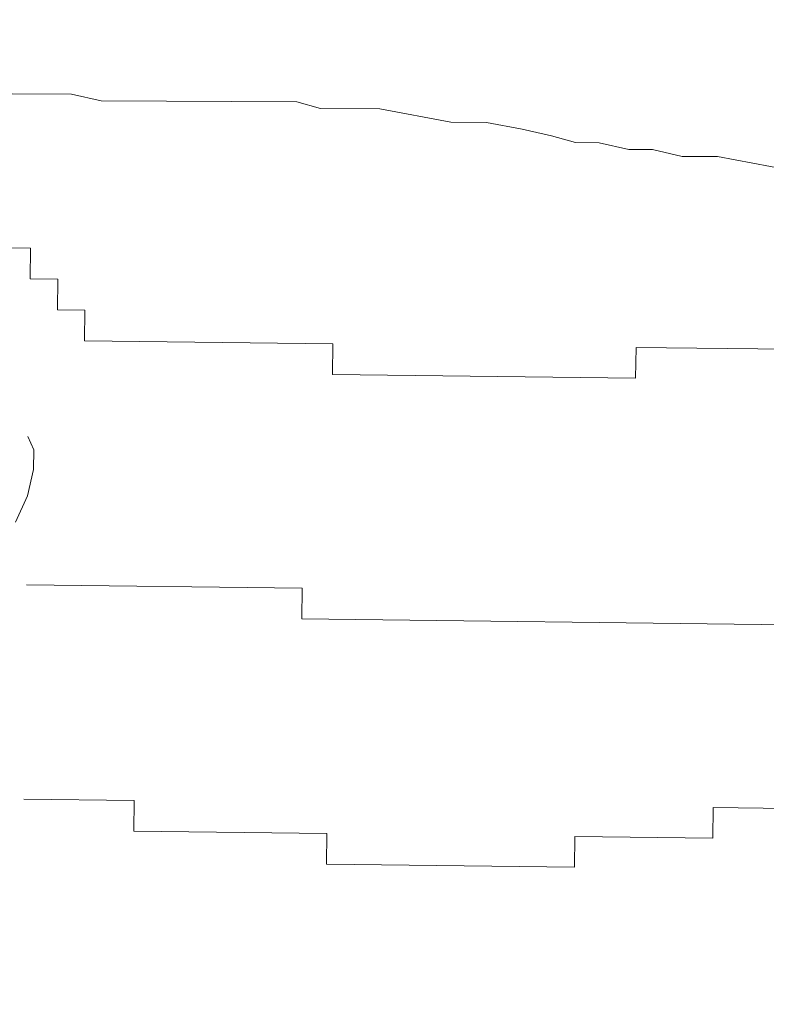
# Model space of a CAD drawing. Units: inches. Extents: x -466983 to 1020, y 324 to 318697.
# Tile 78 of 97: x 652.867 to 656.235, y 944.271 to 948.713. Entities that reach past the tile are written whole.
import ezdxf

# ---------------------------------------------------------------- set-up
doc = ezdxf.new("R2010")
doc.units = ezdxf.units.IN
doc.header["$MEASUREMENT"] = 0
doc.layers.add('A-FLOR-PATT', color=252, linetype='Continuous', lineweight=13)
doc.layers.add('A-FURN', color=8, linetype='Continuous', lineweight=18)

# ---------------------------------------------------------------- blocks, each defined once
blk = doc.blocks.new('L Shaped Sofa')
at = {"ltscale": 2}
for p, q in [((2397.618, 739.4823), (2397.6211, 739.7342)), ((2397.6211, 739.7342), (2399.6627, 739.7093)), ((2399.6627, 739.7093), (2399.6596, 739.4574)), ((2396.4808, 739.2443), (2396.4839, 739.4962)), ((2396.4839, 739.4962), (2397.618, 739.4823)), ((2399.6596, 739.4574), (2401.2474, 739.438)), ((2401.2474, 739.438), (2401.2444, 739.1861)), ((2393.5319, 739.2803), (2396.4808, 739.2443)), ((2401.2444, 739.1861), (2402.1517, 739.175)), ((2395.555, 737.7439), (2399.8649, 737.6912)), ((2399.8649, 737.6912), (2399.8618, 737.4393)), ((2399.8618, 737.4393), (2402.1302, 737.4116)), ((2402.1214, 736.6787), (2402.2204, 736.8951)), ((2402.0713, 736.4621), (2402.1214, 736.6787)), ((2402.0703, 736.2994), (2402.0713, 736.4621)), ((2402.1185, 736.1908), (2402.0703, 736.2994)), ((2397.1151, 735.4573), (2397.1182, 735.7092)), ((2397.1182, 735.7092), (2399.6134, 735.6787)), ((2399.6134, 735.6787), (2399.6103, 735.4268)), ((2394.6199, 735.4878), (2397.1151, 735.4573)), ((2399.6103, 735.4268), (2401.6519, 735.4018)), ((2401.6519, 735.4018), (2401.6488, 735.1499)), ((2401.6488, 735.1499), (2401.8756, 735.1472)), ((2401.8756, 735.1472), (2401.8725, 734.8952)), ((2401.8725, 734.8952), (2402.0994, 734.8925)), ((2402.0994, 734.8925), (2402.0963, 734.6406)), ((2402.0963, 734.6406), (2402.3231, 734.6378)), ((2395.8591, 733.9972), (2396.444, 733.8861)), ((2396.444, 733.8861), (2396.7367, 733.8847)), ((2396.7367, 733.8847), (2396.9804, 733.8293)), ((2396.9804, 733.8293), (2397.1755, 733.8284)), ((2397.1755, 733.8284), (2397.4192, 733.7731)), ((2397.4192, 733.7731), (2397.6144, 733.7721)), ((2397.6144, 733.7721), (2397.8092, 733.717)), ((2397.8092, 733.717), (2398.0529, 733.6616)), ((2398.0529, 733.6616), (2398.3453, 733.6061)), ((2398.3453, 733.6061), (2398.6381, 733.6047)), ((2398.6381, 733.6047), (2399.223, 733.4935)), ((2399.223, 733.4935), (2399.7109, 733.4912)), ((2399.7109, 733.4912), (2399.9058, 733.4361)), ((2399.9058, 733.4361), (2401.516, 733.4285)), ((2401.516, 733.4285), (2401.7596, 733.3732)), ((2401.7596, 733.3732), (2402.2476, 733.3709))]:
    blk.add_line(p, q, dxfattribs=at)

msp = doc.modelspace()

# ---------------------------------------------------------------- hatches: boundary and pattern name
at = {"layer": 'A-FLOR-PATT', "transparency": 33554572}
h = msp.add_hatch(dxfattribs=at)
h.set_pattern_fill('ANSI37', color=256, scale=30)
h.set_pattern_definition([(45, (-1212.4137, -290.035), (-2.6516504, 2.6516504), []), (135, (-1212.4137, -290.035), (-2.6516504, -2.6516504), [])])
h.paths.add_polyline_path([(901.8057, 1075.9377), (900.6144, 1075.9377), (900.6144, 1065.3856), (899.391, 1065.3856), (898.0911, 1065.3856), (892.8356, 1058.7098, -0.258377), (892.1875, 1058.3509), (879.9848, 1058.3509, -0.20177), (879.4382, 1058.5808), (874.0812, 1065.3856), (872.7813, 1065.3856), (871.5579, 1065.3856), (871.5579, 1075.9377), (813.8057, 1075.9377), (813.8057, 1044.7922), (832.3947, 1044.7922, -0.394795), (848.6602, 1028.5356), (848.6602, 1009.9377), (901.8057, 1009.9377), (901.8057, 1015.9377), (901.3057, 1015.9377), (871.3057, 1015.9377), (871.3057, 1017.2502), (871.3344, 1017.2502, -0.401453), (901.3057, 1045.9377), (901.8057, 1045.9377)])
edge = h.paths.add_edge_path(flags=16)
edge.add_line((847.7731, 1068.9486), (847.7731, 1073.7088))
edge.add_arc((849.2269, 1073.7088), 1.4538, 90, 180, ccw=False)
edge.add_line((849.2269, 1075.1627), (864.4921, 1075.1627))
edge.add_arc((864.4921, 1073.7088), 1.4538, 0, 90, ccw=False)
edge.add_line((865.9459, 1073.7088), (865.9459, 1069.0035))
edge.add_arc((832.6447, 1068.9761), 33.3012, -20.61234, 0.04725, ccw=False)
edge.add_ellipse((856.8595, 1058.48), major_axis=(0, 10.2131), ratio=0.6859192, start_angle=100.00884, end_angle=259.99116, ccw=False)
edge.add_arc((881.0742, 1068.9761), 33.3012, 180.04725, 200.61234, ccw=False)
h.paths.add_polyline_path([(853.1456, 1066.4815), (853.1456, 1066.4534), (853.1463, 1066.4534, 0.433107), (852.9166, 1066.6849), (852.9166, 1066.4534), (853.1456, 1066.4534), (853.1456, 1066.4815), (853.088, 1066.6122, 0.697939), (852.6995, 1066.4534), (852.7003, 1066.4534), (852.7003, 1066.4815), (852.9166, 1067.0012), (852.9166, 1066.6849, -0.396254)], flags=0)
h.paths.add_polyline_path([(861.0187, 1066.4815), (861.0187, 1066.4534), (861.0194, 1066.4534, 0.416404), (860.8024, 1066.6849), (860.8024, 1066.4534), (861.0187, 1066.4534), (861.0187, 1066.4815), (860.9672, 1066.6053, 0.713344), (860.5726, 1066.4534), (860.5734, 1066.4534), (860.5734, 1066.4815), (860.8024, 1067.0012), (860.8024, 1066.6849, -0.379973)], flags=0)
edge = h.paths.add_edge_path(flags=0)
edge.add_spline(control_points=[(861.1298, 1065.7855), (861.4661, 1065.2478), (861.6134, 1065.0161), (861.9833, 1064.3736), (862.1924, 1063.9443), (862.5614, 1063.0391), (862.7212, 1062.5633), (862.9865, 1061.5781), (863.092, 1061.0689), (863.2452, 1060.031), (863.293, 1059.5025), (863.3295, 1058.4409), (863.3181, 1057.9078), (863.2366, 1056.8518), (863.1664, 1056.3289), (862.9695, 1055.308), (862.8427, 1054.8099), (862.5365, 1053.8522), (862.3571, 1053.3927), (861.9514, 1052.5249), (861.7251, 1052.1166), (861.233, 1051.3622), (860.9672, 1051.0162), (860.4048, 1050.3949), (860.1082, 1050.1197), (859.4937, 1049.6461), (859.1758, 1049.4476), (858.5276, 1049.1299), (858.1973, 1049.0107), (857.5315, 1048.8518), (857.1959, 1048.8121), (856.5249, 1048.812), (856.1894, 1048.8515), (855.5236, 1049.0101), (855.1933, 1049.1291), (854.545, 1049.4465), (854.2271, 1049.6449), (853.6124, 1050.1183), (853.3158, 1050.3933), (852.7533, 1051.0143), (852.4874, 1051.3602), (851.9952, 1052.1144), (851.7688, 1052.5225), (851.3629, 1053.3902), (851.1834, 1053.8496), (850.877, 1054.8071), (850.7501, 1055.3051), (850.553, 1056.326), (850.4827, 1056.8488), (850.401, 1057.9048), (850.3895, 1058.4379), (850.4257, 1059.4995), (850.4734, 1060.0281), (850.6265, 1061.066), (850.7318, 1061.5753), (850.9969, 1062.5605), (851.1567, 1063.0365), (851.5254, 1063.9418), (851.7345, 1064.3712), (852.1056, 1065.0164), (852.2544, 1065.2503), (852.6082, 1065.7335)], knot_values=[3.915332, 3.915332, 3.915332, 3.915332, 4.013468, 4.013468, 4.175532, 4.175532, 4.337596, 4.337596, 4.49966, 4.49966, 4.661724, 4.661724, 4.823788, 4.823788, 4.985852, 4.985852, 5.147916, 5.147916, 5.30998, 5.30998, 5.472044, 5.472044, 5.634109, 5.634109, 5.796173, 5.796173, 5.958237, 5.958237, 6.120301, 6.120301, 6.282365, 6.282365, 6.444429, 6.444429, 6.606493, 6.606493, 6.768557, 6.768557, 6.930621, 6.930621, 7.092685, 7.092685, 7.254749, 7.254749, 7.416813, 7.416813, 7.578878, 7.578878, 7.740942, 7.740942, 7.903006, 7.903006, 8.06507, 8.06507, 8.227134, 8.227134, 8.389198, 8.389198, 8.551262, 8.551262, 8.65037, 8.65037, 8.65037, 8.65037], degree=3, periodic=0)
edge.add_line((852.6421, 1065.7855), (861.1298, 1065.7855))
edge = h.paths.add_edge_path(flags=0)
edge.add_ellipse((856.8496, 1057.7432), major_axis=(0, 7.7921), ratio=0.687861, start_angle=0, end_angle=360)
h.paths.add_polyline_path([(848.8634, 1069.3891), (848.8634, 1073.9605, -0.414214), (849.9538, 1075.0508), (863.7652, 1075.0508, -0.414214), (864.8555, 1073.9605), (864.8555, 1069.3891, -0.388936), (864.5237, 1069.027, -0.043561), (849.1953, 1069.027, -0.388936)], flags=0)
h.paths.add_polyline_path([(853.1006, 1068.1122, -1), (852.6775, 1068.1122, -1)], flags=0)
edge = h.paths.add_edge_path(flags=0)
edge.add_ellipse((856.8595, 1057.3378), major_axis=(0, 2.207), ratio=0.657164, start_angle=0, end_angle=360)
h.paths.add_polyline_path([(861.0415, 1068.1122, -1), (860.6184, 1068.1122, -1)], flags=0)
edge = h.paths.add_edge_path()
edge.add_line((573.9537, 1057.3412), (573.9537, 1075.9377))
edge.add_line((573.9537, 1075.9377), (558.7308, 1075.9377))
edge.add_line((558.7308, 1075.9377), (558.7308, 1065.3856))
edge.add_line((558.7308, 1065.3856), (557.5074, 1065.3856))
edge.add_line((557.5074, 1065.3856), (556.2075, 1065.3856))
edge.add_line((556.2075, 1065.3856), (550.952, 1058.7098))
edge.add_arc((550.3039, 1059.1155), 0.7646, 270, 327.9483, ccw=False)
edge.add_line((550.3039, 1058.3509), (538.1012, 1058.3509))
edge.add_arc((538.1012, 1059.1155), 0.7646, 224.3704, 270, ccw=False)
edge.add_line((537.5546, 1058.5808), (532.1976, 1065.3856))
edge.add_line((532.1976, 1065.3856), (530.8977, 1065.3856))
edge.add_line((530.8977, 1065.3856), (529.6743, 1065.3856))
edge.add_line((529.6743, 1065.3856), (529.6743, 1075.9377))
edge.add_line((529.6743, 1075.9377), (520.8057, 1075.9377))
edge.add_line((520.8057, 1075.9377), (520.8057, 1045.9377))
edge.add_line((520.8057, 1045.9377), (521.3057, 1045.9377))
edge.add_arc((521.3057, 1015.9377), 30, 2.50749, 90, ccw=False)
edge.add_line((551.277, 1017.2502), (551.3057, 1017.2502))
edge.add_line((551.3057, 1017.2502), (551.3057, 1015.9377))
edge.add_line((551.3057, 1015.9377), (520.8057, 1015.9377))
edge.add_line((520.8057, 1015.9377), (520.8057, 1009.9377))
edge.add_line((520.8057, 1009.9377), (559.1913, 1010.4022))
edge.add_arc((559.1913, 1011.856), 1.4538, 180, 270, ccw=False)
edge.add_line((557.7375, 1011.856), (557.7375, 1016.5613))
edge.add_arc((591.0386, 1016.5888), 33.3012, 159.38766, 180.04725, ccw=False)
edge.add_ellipse((566.8239, 1027.0848), major_axis=(0, 10.2131), ratio=0.6859192, start_angle=280.00884, end_angle=439.99116, ccw=False)
edge.add_arc((542.6091, 1016.5888), 33.3012, 0.04725, 20.61234, ccw=False)
edge.add_line((575.9103, 1016.6162), (575.9103, 1011.856))
edge.add_arc((574.4565, 1011.856), 1.4538, -90, 0, ccw=False)
edge.add_line((574.4565, 1010.4022), (608.8057, 1009.9377))
edge.add_line((608.8057, 1009.9377), (608.8057, 1041.0857))
edge.add_line((608.8057, 1041.0857), (590.2179, 1041.0857))
edge.add_arc((590.775, 1057.9074), 16.8309, 181.92775, 268.10321, ccw=False)
edge = h.paths.add_edge_path()
edge.add_ellipse((494.2443, 583.6204), major_axis=(0, 10.2131), ratio=0.6859192, start_angle=280.00884, end_angle=439.99116, ccw=False)
edge.add_arc((470.0296, 573.1243), 33.3012, 0.04725, 20.61234, ccw=False)
edge.add_line((503.3307, 573.1518), (503.3307, 568.3916))
edge.add_arc((501.8769, 568.3916), 1.4538, -90, 0, ccw=False)
edge.add_line((501.8769, 566.9377), (539.8057, 566.9377))
edge.add_line((539.8057, 566.9377), (539.8057, 572.9377))
edge.add_line((539.8057, 572.9377), (539.3057, 572.9377))
edge.add_line((539.3057, 572.9377), (509.3057, 572.9377))
edge.add_line((509.3057, 572.9377), (509.3057, 574.2502))
edge.add_line((509.3057, 574.2502), (509.3344, 574.2502))
edge.add_arc((539.3057, 572.9377), 30, 90, 177.49251, ccw=False)
edge.add_line((539.3057, 602.9377), (539.8057, 602.9377))
edge.add_line((539.8057, 602.9377), (539.8057, 626.9377))
edge.add_line((539.8057, 626.9377), (531.7718, 626.9377))
edge.add_line((531.7718, 626.9377), (531.7718, 616.3856))
edge.add_line((531.7718, 616.3856), (530.5484, 616.3856))
edge.add_line((530.5484, 616.3856), (529.2485, 616.3856))
edge.add_line((529.2485, 616.3856), (523.7105, 609.3509))
edge.add_line((523.7105, 609.3509), (510.7766, 609.3509))
edge.add_line((510.7766, 609.3509), (505.2386, 616.3856))
edge.add_line((505.2386, 616.3856), (503.9387, 616.3856))
edge.add_line((503.9387, 616.3856), (502.7153, 616.3856))
edge.add_line((502.7153, 616.3856), (502.7153, 626.9377))
edge.add_line((502.7153, 626.9377), (481.6983, 626.9377))
edge.add_line((481.6983, 626.9377), (481.6983, 610.995))
edge.add_arc((467.2703, 611.4728), 14.4359, 271.92775, 358.10321, ccw=False)
edge.add_line((467.7559, 597.0451), (451.8057, 597.0451))
edge.add_line((451.8057, 597.0451), (451.8057, 584.4035))
edge.add_line((451.8057, 584.4035), (451.8057, 566.9377))
edge.add_line((451.8057, 566.9377), (486.6117, 566.9377))
edge.add_arc((486.6117, 568.3916), 1.4538, 180, 270, ccw=False)
edge.add_line((485.1579, 568.3916), (485.1579, 573.0969))
edge.add_arc((518.4591, 573.1243), 33.3012, 159.38766, 180.04725, ccw=False)
h.paths.add_polyline_path([(836.2609, 1020.7328), (879.8898, 1020.7328), (879.8898, 1039.3902), (836.2609, 1039.3902)], flags=25)
h.paths.add_polyline_path([(549.9851, 1036.7492), (593.614, 1036.7492), (593.614, 1055.4065), (549.9851, 1055.4065)], flags=24)
h.paths.add_polyline_path([(475.123, 595.5959), (518.752, 595.5959), (518.752, 614.2532), (475.123, 614.2532)], flags=24)
h = msp.add_hatch(dxfattribs=at)
h.set_pattern_fill('ANSI37', color=256, scale=20)
h.set_pattern_definition([(45, (-1212.4137, -290.035), (-1.767767, 1.767767), []), (135, (-1212.4137, -290.035), (-1.767767, -1.767767), [])])
h.paths.add_polyline_path([(809.8057, 870.9377), (809.8057, 888.1519), (806.9985, 888.1519), (802.6624, 888.1519), (789.3832, 888.1519), (786.2846, 888.1519, -0.414214), (785.4991, 888.9374), (785.4991, 900.1959), (785.4991, 908.4696, -0.414214), (786.8082, 909.7787, -0.414214), (785.4991, 911.0878), (785.4991, 929.1015, -0.414214), (786.8082, 930.4106, -0.414214), (785.4991, 931.7197), (785.4991, 931.9039, -0.414214), (784.19, 930.5948), (766.7223, 930.5948, -0.412359), (765.4132, 931.8956, -0.413741), (764.1145, 930.5782), (744.5781, 930.422, -0.416556), (743.7864, 931.2075), (743.7864, 933.5153), (742.2154, 933.5153), (742.2154, 952.024, -0.001344), (743.7864, 952.1998), (743.7864, 953.9377), (678.5915, 953.9377), (678.5915, 951.1305), (678.5915, 946.7945), (678.5915, 933.5153), (678.5915, 930.4166, -0.414214), (677.806, 929.6312), (666.5475, 929.6312), (658.2738, 929.6312, -0.414214), (656.9647, 930.9403, -0.414214), (655.6556, 929.6312), (637.6419, 929.6312, -0.414214), (636.3328, 930.9403, -0.414214), (635.0237, 929.6312), (634.8395, 929.6312, -0.414214), (636.1486, 928.322), (636.1486, 910.8544, -0.412359), (634.8478, 909.5452, -0.413741), (636.1653, 908.2466), (636.3214, 888.7102, -0.416556), (635.5359, 887.9184), (633.2281, 887.9184), (633.2281, 886.3475), (614.7194, 886.3475, -0.001344), (614.5436, 887.9184), (612.8057, 887.9184), (612.8057, 834.9377), (612.8057, 752.9377), (612.8057, 748.9377), (612.8057, 697.9377), (654.8057, 697.9377), (654.8057, 701.9377), (715.8057, 701.9377), (715.8057, 737.4353), (774.2918, 737.4353), (774.2918, 795.9377), (809.8057, 795.9377)])
h.paths.add_polyline_path([(679.2761, 849.5757, 0.102523), (682.1475, 849.2608, -0.080461), (694.5428, 849.7725, -0.283899), (694.4822, 849.0082, 0.136605), (694.4068, 848.8103, -0.030441), (694.5428, 846.8929), (694.5428, 842.6198), (694.5428, 838.3466, -0.028219), (694.4246, 836.5684), (694.425, 836.5684, 0.196187), (694.4456, 836.2708, -0.302897), (694.5428, 835.467, -0.080461), (682.1475, 835.9787, 0.102523), (679.2761, 835.6638, -0.58611), (678.6457, 836.0169), (678.6457, 849.2227, -0.58611)], flags=16)
h.paths.add_polyline_path([(679.5173, 848.6515, 0.699597), (679.476, 848.6342, 1.20716), (679.1935, 848.7422, 0.010621)], flags=0)
h.paths.add_polyline_path([(679.4923, 836.5608, -0.013798), (679.9178, 836.6594, -0.071703), (682.8533, 837.1434, -0.165743), (682.1665, 839.1006), (682.1665, 842.6094), (682.1665, 846.0603, -0.240616), (683.4733, 848.6767, -0.068263), (693.9295, 849.0082), (693.7875, 848.7083), (693.7875, 849.0228, 0.067332), (683.4733, 848.6767, 0.240616), (682.1665, 846.0603), (682.1665, 842.6094), (682.1665, 839.1006, 0.23459), (683.461, 836.5513, 0.068093), (693.7875, 836.1955), (693.7875, 836.5104), (693.9296, 836.2102, -0.077215), (682.2421, 836.7815, 0.086627), (679.5283, 836.5701, -0.628402), (679.5029, 836.5735), (679.5029, 836.6071, 0.910458)], flags=0)
h.paths.add_polyline_path([(679.476, 848.6364), (679.2069, 848.647), (679.2069, 836.5718, 0.913566), (679.3645, 836.5861), (679.476, 836.5824)], flags=0)
h.paths.add_polyline_path([(679.2761, 829.8604, 0.102523), (682.1475, 829.5455, -0.080461), (694.5428, 830.0572, -0.283899), (694.4822, 829.2929, 0.136605), (694.4068, 829.095, -0.030441), (694.5428, 827.1776), (694.5428, 822.9045), (694.5428, 818.6314, -0.028219), (694.4246, 816.8531), (694.425, 816.8532, 0.196187), (694.4456, 816.5555, -0.302897), (694.5428, 815.7517, -0.080461), (682.1475, 816.2635, 0.102523), (679.2761, 815.9485, -0.58611), (678.6457, 816.3016), (678.6457, 829.5074, -0.58611)], flags=16)
h.paths.add_polyline_path([(679.5173, 828.9362, 0.699597), (679.476, 828.9189, 1.20716), (679.1935, 829.0269, 0.010621)], flags=0)
h.paths.add_polyline_path([(679.4923, 816.8456, -0.013798), (679.9178, 816.9441, -0.071703), (682.8533, 817.4281, -0.165743), (682.1665, 819.3853), (682.1665, 822.8941), (682.1665, 826.345, -0.240616), (683.4733, 828.9614, -0.068263), (693.9295, 829.2929), (693.7875, 828.9931), (693.7875, 829.3076, 0.067332), (683.4733, 828.9614, 0.240616), (682.1665, 826.345), (682.1665, 822.8941), (682.1665, 819.3853, 0.23459), (683.461, 816.836, 0.068093), (693.7875, 816.4802), (693.7875, 816.7952), (693.9296, 816.4949, -0.077215), (682.2421, 817.0662, 0.086627), (679.5283, 816.8549, -0.628402), (679.5029, 816.8582), (679.5029, 816.8918, 0.910458)], flags=0)
h.paths.add_polyline_path([(679.476, 828.9211), (679.2069, 828.9317), (679.2069, 816.8565, 0.913566), (679.3645, 816.8708), (679.476, 816.8671)], flags=0)
h.paths.add_polyline_path([(679.2761, 810.1451, 0.102523), (682.1475, 809.8302, -0.080461), (694.5428, 810.342, -0.3023), (694.4466, 809.5394, 0.10023), (694.4058, 809.3878, -0.03057), (694.5428, 807.4623), (694.5428, 803.1892), (694.5428, 798.9161, -0.03057), (694.4058, 796.9906, 0.10023), (694.4466, 796.839, -0.3023), (694.5428, 796.0365, -0.080461), (682.1475, 796.5482, 0.102523), (679.2761, 796.2333, -0.58611), (678.6457, 796.5863), (678.6457, 809.7921, -0.58611)], flags=16)
h.paths.add_polyline_path([(679.5173, 809.2417, 0.699597), (679.476, 809.2244, 1.20716), (679.1935, 809.3324, 0.010621)], flags=0)
h.paths.add_polyline_path([(679.4923, 797.151, -0.013798), (679.9178, 797.2496, -0.071703), (682.8533, 797.7336, -0.165743), (682.1665, 799.6908), (682.1665, 803.1996), (682.1665, 806.6505, -0.239349), (683.461, 809.2577, -0.072465), (694.4468, 809.5405, 0.197932), (694.425, 809.2405), (693.7875, 809.2985), (693.7875, 809.6135, 0.068093), (683.461, 809.2577, 0.239349), (682.1665, 806.6505), (682.1665, 803.1996), (682.1665, 799.6908, 0.235854), (683.4733, 797.1323, 0.067332), (693.7875, 796.7861), (693.7875, 797.1006), (694.425, 797.1586, 0.197932), (694.4468, 796.8586, -0.080419), (682.1557, 797.3795, 0.083867), (679.5283, 797.1603, -0.628402), (679.5029, 797.1637), (679.5029, 797.1973, 0.910458)], flags=0)
h.paths.add_polyline_path([(679.2069, 809.2372), (679.2069, 797.162, 0.913566), (679.3645, 797.1763), (679.476, 797.1726), (679.476, 809.2266)], flags=0)
h.paths.add_polyline_path([(695.3643, 853.2989), (728.2231, 853.2989), (728.2231, 771.1519), (695.3643, 771.1519)], flags=16)
h.paths.add_polyline_path([(696.0215, 852.6417), (727.5659, 852.6417), (727.5659, 771.809), (696.0215, 771.809)], flags=0)
h.paths.add_polyline_path([(679.2761, 788.7869, 0.102523), (682.1475, 788.472, -0.080461), (694.5428, 788.9837, -0.3023), (694.4466, 788.1812, 0.10023), (694.4058, 788.0296, -0.03057), (694.5428, 786.1041), (694.5428, 781.831), (694.5428, 777.5578, -0.03057), (694.4058, 775.6323, 0.10023), (694.4466, 775.4808, -0.3023), (694.5428, 774.6782, -0.080461), (682.1475, 775.19, 0.102523), (679.2761, 774.875, -0.58611), (678.6457, 775.2281), (678.6457, 788.4339, -0.58611)], flags=16)
h.paths.add_polyline_path([(679.5173, 787.8834, 0.699597), (679.476, 787.8662, 1.20716), (679.1935, 787.9742, 0.010621)], flags=0)
h.paths.add_polyline_path([(679.4923, 775.7928, -0.013798), (679.9178, 775.8914, -0.071703), (682.8533, 776.3753, -0.165743), (682.1665, 778.3325), (682.1665, 781.8414), (682.1665, 785.2922, -0.239349), (683.461, 787.8995, -0.072465), (694.4468, 788.1823, 0.197932), (694.425, 787.8823), (693.7875, 787.9403), (693.7875, 788.2553, 0.068093), (683.461, 787.8995, 0.239349), (682.1665, 785.2922), (682.1665, 781.8414), (682.1665, 778.3325, 0.235854), (683.4733, 775.7741, 0.067332), (693.7875, 775.4279), (693.7875, 775.7424), (694.425, 775.8004, 0.197932), (694.4468, 775.5004, -0.080419), (682.1557, 776.0212, 0.083867), (679.5283, 775.8021, -0.628402), (679.5029, 775.8054), (679.5029, 775.8391, 0.910458)], flags=0)
h.paths.add_polyline_path([(679.2069, 787.8789), (679.2069, 775.8038, 0.913566), (679.3645, 775.818), (679.476, 775.8144), (679.476, 787.8684)], flags=0)
h.paths.add_polyline_path([(704.641, 854.1204, -0.080461), (705.1527, 866.5157, 0.102523), (704.8378, 869.3871, -0.58611), (705.1908, 870.0174), (718.3966, 870.0174, -0.58611), (718.7496, 869.3871, 0.102523), (718.4347, 866.5157, -0.080461), (718.9465, 854.1204, -0.3023), (718.1439, 854.2166, 0.10023), (717.9924, 854.2574, -0.03057), (716.0668, 854.1204), (711.7937, 854.1204), (707.5206, 854.1204, -0.03057), (705.5951, 854.2574, 0.10023), (705.4435, 854.2166, -0.3023)], flags=16)
h.paths.add_polyline_path([(717.8462, 869.1459, 0.699597), (717.8289, 869.1872, 1.20716), (717.9369, 869.4697, 0.010621)], flags=0)
h.paths.add_polyline_path([(705.4631, 854.2164, -0.080419), (705.984, 866.5074, 0.083867), (705.7648, 869.1349, -0.628402), (705.7682, 869.1603), (705.8018, 869.1603, 0.910458), (705.7555, 869.1709, -0.013798), (705.8541, 868.7454, -0.071703), (706.3381, 865.8099, -0.165743), (708.2953, 866.4967), (711.8041, 866.4967), (715.255, 866.4967, -0.239349), (717.8622, 865.2022, -0.072465), (718.145, 854.2164, 0.197932), (717.845, 854.2382), (717.903, 854.8757), (718.218, 854.8757, 0.068093), (717.8622, 865.2022, 0.239349), (715.255, 866.4967), (711.8041, 866.4967), (708.2953, 866.4967, 0.235854), (705.7368, 865.1898, 0.067332), (705.3906, 854.8757), (705.7051, 854.8757), (705.7631, 854.2382, 0.197932)], flags=16)
h.paths.add_polyline_path([(705.7665, 869.4563, 0.913566), (705.7808, 869.2987), (705.7771, 869.1872), (717.8311, 869.1872), (717.8417, 869.4563)], flags=0)
h.paths.add_polyline_path([(729.0446, 842.6198), (729.0446, 846.8929, -0.03057), (729.1817, 848.8184, 0.10023), (729.1408, 848.9699, -0.3023), (729.0446, 849.7725, -0.080461), (741.4399, 849.2608, 0.102523), (744.3113, 849.5757, -0.58611), (744.9417, 849.2227), (744.9417, 836.0169, -0.58611), (744.3113, 835.6638, 0.102523), (741.4399, 835.9787, -0.080461), (729.0446, 835.467, -0.3023), (729.1408, 836.2696, 0.10023), (729.1817, 836.4211, -0.03057), (729.0446, 838.3466)], flags=16)
h.paths.add_polyline_path([(744.1115, 836.5846, 1.20716), (744.3939, 836.4766, 0.010621), (744.0701, 836.5673, 0.699597)], flags=0)
h.paths.add_polyline_path([(729.1407, 836.2684, 0.197932), (729.1624, 836.5684), (729.7999, 836.5104), (729.7999, 836.1955, 0.068093), (740.1264, 836.5513, 0.239349), (741.4209, 839.1585), (741.4209, 842.6094), (741.4209, 846.1182, 0.235854), (740.1141, 848.6767, 0.067332), (729.7999, 849.0228), (729.7999, 848.7083), (729.1624, 848.6503, 0.197932), (729.1407, 848.9504, -0.080419), (741.4317, 848.4295, 0.083867), (744.0591, 848.6486, -0.628402), (744.0845, 848.6453), (744.0845, 848.6117, 0.910458), (744.0951, 848.6579, -0.013798), (743.6696, 848.5594, -0.071703), (740.7341, 848.0754, -0.165743), (741.4209, 846.1182), (741.4209, 842.6094), (741.4209, 839.1585, -0.239349), (740.1264, 836.5513, -0.072465)], flags=0)
h.paths.add_polyline_path([(729.0446, 830.0572, -0.080461), (741.4399, 829.5455, 0.102523), (744.3113, 829.8604, -0.58611), (744.9417, 829.5074), (744.9417, 816.3016, -0.58611), (744.3113, 815.9485, 0.102523), (741.4399, 816.2635, -0.080461), (729.0446, 815.7517, -0.3023), (729.1408, 816.5543, 0.10023), (729.1817, 816.7058, -0.03057), (729.0446, 818.6314), (729.0446, 822.9045), (729.0446, 827.1776, -0.03057), (729.1817, 829.1031, 0.10023), (729.1408, 829.2547, -0.3023)], flags=16)
h.paths.add_polyline_path([(744.1115, 816.8693, 1.20716), (744.3939, 816.7613, 0.010621), (744.0701, 816.852, 0.699597)], flags=0)
h.paths.add_polyline_path([(729.1407, 829.2351, -0.080419), (741.4317, 828.7142, 0.083867), (744.0591, 828.9334, -0.628402), (744.0845, 828.93), (744.0845, 828.8964, 0.910458), (744.0951, 828.9427, -0.013798), (743.6696, 828.8441, -0.071703), (740.7341, 828.3601, -0.165743), (741.4209, 826.4029), (741.4209, 822.8941), (741.4209, 819.4432, -0.239349), (740.1264, 816.836, -0.072465), (729.1407, 816.5531, 0.197932), (729.1624, 816.8532), (729.7999, 816.7952), (729.7999, 816.4802, 0.068093), (740.1264, 816.836, 0.239349), (741.4209, 819.4432), (741.4209, 822.8941), (741.4209, 826.4029, 0.235854), (740.1141, 828.9614, 0.067332), (729.7999, 829.3076), (729.7999, 828.9931), (729.1624, 828.9351, 0.197932)], flags=16)
h.paths.add_polyline_path([(729.0446, 810.342, -0.080461), (741.4399, 809.8302, 0.102523), (744.3113, 810.1451, -0.58611), (744.9417, 809.7921), (744.9417, 796.5863, -0.58611), (744.3113, 796.2333, 0.102523), (741.4399, 796.5482, -0.080461), (729.0446, 796.0365, -0.283899), (729.1052, 796.8007, 0.136605), (729.1806, 796.9987, -0.030441), (729.0446, 798.9161), (729.0446, 803.1892), (729.0446, 807.4623, -0.028219), (729.1628, 809.2406), (729.1624, 809.2405, 0.196187), (729.1418, 809.5382, -0.302897)], flags=16)
h.paths.add_polyline_path([(744.1115, 797.1748, 1.20716), (744.3939, 797.0668, 0.010621), (744.0701, 797.1575, 0.699597)], flags=0)
h.paths.add_polyline_path([(741.3453, 809.0275, 0.086627), (744.0591, 809.2388, -0.628402), (744.0845, 809.2355), (744.0845, 809.2019, 0.910458), (744.0951, 809.2481, -0.013798), (743.6696, 809.1496, -0.071703), (740.7341, 808.6656, -0.165743), (741.4209, 806.7084), (741.4209, 803.1996), (741.4209, 799.7487, -0.240616), (740.1141, 797.1323, -0.068263), (729.658, 796.8008), (729.7999, 797.1006), (729.7999, 796.7861, 0.067332), (740.1141, 797.1323, 0.240616), (741.4209, 799.7487), (741.4209, 803.1996), (741.4209, 806.7084, 0.23459), (740.1264, 809.2577, 0.068093), (729.7999, 809.6135), (729.7999, 809.2985), (729.6578, 809.5988, -0.077215)], flags=0)
h.paths.add_polyline_path([(704.641, 770.3304, -0.283899), (705.4053, 770.2697, 0.136605), (705.6032, 770.1944, -0.030441), (707.5206, 770.3304), (711.7937, 770.3304), (716.0668, 770.3304, -0.028219), (717.8451, 770.2122), (717.845, 770.2126, 0.196187), (718.1427, 770.2331, -0.302897), (718.9465, 770.3304, -0.080461), (718.4347, 757.9351, 0.102523), (718.7496, 755.0637, -0.58611), (718.3966, 754.4333), (705.1908, 754.4333, -0.58611), (704.8378, 755.0637, 0.102523), (705.1527, 757.9351, -0.080461)], flags=16)
h.paths.add_polyline_path([(705.762, 755.3048, 0.699597), (705.7793, 755.2635, 1.20716), (705.6713, 754.9811, 0.010621)], flags=0)
h.paths.add_polyline_path([(705.4053, 769.717), (705.7051, 769.5751), (705.3906, 769.5751, 0.067332), (705.7368, 759.2609, 0.240616), (708.3532, 757.954), (711.8041, 757.954), (715.3129, 757.954, 0.23459), (717.8622, 759.2485, 0.068093), (718.218, 769.5751), (717.903, 769.5751), (718.2033, 769.7172, -0.077215), (717.632, 758.0297, 0.086627), (717.8433, 755.3159, -0.628402), (717.84, 755.2904), (717.8064, 755.2904, 0.910458), (717.8526, 755.2799, -0.013798), (717.7541, 755.7053, -0.071703), (717.2701, 758.6409, -0.165743), (715.3129, 757.954), (711.8041, 757.954), (708.3532, 757.954, -0.240616), (705.7368, 759.2609, -0.068263)], flags=0)
h.paths.add_polyline_path([(729.0446, 788.9837, -0.080461), (741.4399, 788.472, 0.102523), (744.3113, 788.7869, -0.58611), (744.9417, 788.4339), (744.9417, 775.2281, -0.58611), (744.3113, 774.875, 0.102523), (741.4399, 775.19, -0.080461), (729.0446, 774.6782, -0.283899), (729.1052, 775.4425, 0.136605), (729.1806, 775.6405, -0.030441), (729.0446, 777.5578), (729.0446, 781.831), (729.0446, 786.1041, -0.028219), (729.1628, 787.8823), (729.1624, 787.8823, 0.196187), (729.1418, 788.1799, -0.302897)], flags=16)
h.paths.add_polyline_path([(744.1115, 775.8165, 1.20716), (744.3939, 775.7086, 0.010621), (744.0701, 775.7993, 0.699597)], flags=0)
h.paths.add_polyline_path([(741.3453, 787.6692, 0.086627), (744.0591, 787.8806, -0.628402), (744.0845, 787.8773), (744.0845, 787.8437, 0.910458), (744.0951, 787.8899, -0.013798), (743.6696, 787.7913, -0.071703), (740.7341, 787.3074, -0.165743), (741.4209, 785.3502), (741.4209, 781.8414), (741.4209, 778.3905, -0.240616), (740.1141, 775.7741, -0.068263), (729.658, 775.4425), (729.7999, 775.7424), (729.7999, 775.4279, 0.067332), (740.1141, 775.7741, 0.240616), (741.4209, 778.3905), (741.4209, 781.8414), (741.4209, 785.3502, 0.23459), (740.1264, 787.8995, 0.068093), (729.7999, 788.2553), (729.7999, 787.9403), (729.6578, 788.2405, -0.077215)], flags=0)
h.paths.add_polyline_path([(744.1115, 848.6364), (744.1115, 836.5824), (744.3805, 836.5718), (744.3805, 848.647, 0.913566), (744.2229, 848.6327)], flags=0)
h.paths.add_polyline_path([(744.2229, 828.9174), (744.1115, 828.9211), (744.1115, 816.8671), (744.3805, 816.8565), (744.3805, 828.9317, 0.913566)], flags=0)
h.paths.add_polyline_path([(717.8311, 755.2635), (705.7771, 755.2635), (705.7665, 754.9945), (717.8417, 754.9945, 0.913566), (717.8274, 755.1521)], flags=0)
h.paths.add_polyline_path([(744.2229, 809.2229), (744.1115, 809.2266), (744.1115, 797.1726), (744.3805, 797.162), (744.3805, 809.2372, 0.913566)], flags=0)
h.paths.add_polyline_path([(744.1115, 787.8684), (744.1115, 775.8144), (744.3805, 775.8038), (744.3805, 787.8789, 0.913566), (744.2229, 787.8647)], flags=0)
h.paths.add_polyline_path([(678.8774, 877.1228), (737.6127, 877.1228), (737.6127, 899.5116), (678.8774, 899.5116)], flags=24)

# ---------------------------------------------------------------- linework, layer by layer
at = {"layer": 'A-FURN', "ltscale": 2}
for p, q in [((653.1012, 948.3768), (652.8337, 948.378)), ((653.1012, 948.3768), (652.8337, 948.378)), ((653.1012, 948.3768), (652.8337, 948.378)), ((653.1012, 948.3768), (652.8337, 948.378)), ((653.1012, 948.3768), (652.8337, 948.378)), ((653.1012, 948.3768), (652.8337, 948.378)), ((653.2348, 948.3464), (653.1012, 948.3768)), ((653.2348, 948.3464), (653.1012, 948.3768)), ((653.2348, 948.3464), (653.1012, 948.3768)), ((653.2348, 948.3464), (653.1012, 948.3768)), ((653.2348, 948.3464), (653.1012, 948.3768)), ((653.2348, 948.3464), (653.1012, 948.3768)), ((654.1176, 948.3423), (653.2348, 948.3464)), ((654.1176, 948.3423), (653.2348, 948.3464)), ((654.1176, 948.3423), (653.2348, 948.3464)), ((654.1176, 948.3423), (653.2348, 948.3464)), ((654.1176, 948.3423), (653.2348, 948.3464)), ((654.1176, 948.3423), (653.2348, 948.3464)), ((654.2244, 948.3121), (654.1176, 948.3423)), ((654.2244, 948.3121), (654.1176, 948.3423)), ((654.2244, 948.3121), (654.1176, 948.3423)), ((654.2244, 948.3121), (654.1176, 948.3423)), ((654.2244, 948.3121), (654.1176, 948.3423)), ((654.2244, 948.3121), (654.1176, 948.3423)), ((654.4919, 948.3108), (654.2244, 948.3121)), ((654.4919, 948.3108), (654.2244, 948.3121)), ((654.4919, 948.3108), (654.2244, 948.3121)), ((654.4919, 948.3108), (654.2244, 948.3121)), ((654.4919, 948.3108), (654.2244, 948.3121)), ((654.4919, 948.3108), (654.2244, 948.3121)), ((654.8125, 948.2498), (654.4919, 948.3108)), ((654.8125, 948.2498), (654.4919, 948.3108)), ((654.8125, 948.2498), (654.4919, 948.3108)), ((654.8125, 948.2498), (654.4919, 948.3108)), ((654.8125, 948.2498), (654.4919, 948.3108)), ((654.8125, 948.2498), (654.4919, 948.3108)), ((654.973, 948.2491), (654.8125, 948.2498)), ((654.973, 948.2491), (654.8125, 948.2498)), ((654.973, 948.2491), (654.8125, 948.2498)), ((654.973, 948.2491), (654.8125, 948.2498)), ((654.973, 948.2491), (654.8125, 948.2498)), ((654.973, 948.2491), (654.8125, 948.2498)), ((655.1334, 948.2186), (654.973, 948.2491)), ((655.1334, 948.2186), (654.973, 948.2491)), ((655.1334, 948.2186), (654.973, 948.2491)), ((655.1334, 948.2186), (654.973, 948.2491)), ((655.1334, 948.2186), (654.973, 948.2491)), ((655.1334, 948.2186), (654.973, 948.2491)), ((655.2669, 948.1883), (655.1334, 948.2186)), ((655.2669, 948.1883), (655.1334, 948.2186)), ((655.2669, 948.1883), (655.1334, 948.2186)), ((655.2669, 948.1883), (655.1334, 948.2186)), ((655.2669, 948.1883), (655.1334, 948.2186)), ((655.2669, 948.1883), (655.1334, 948.2186)), ((655.3737, 948.158), (655.2669, 948.1883)), ((655.3737, 948.158), (655.2669, 948.1883)), ((655.3737, 948.158), (655.2669, 948.1883)), ((655.3737, 948.158), (655.2669, 948.1883)), ((655.3737, 948.158), (655.2669, 948.1883)), ((655.3737, 948.158), (655.2669, 948.1883)), ((655.4807, 948.1575), (655.3737, 948.158)), ((655.4807, 948.1575), (655.3737, 948.158)), ((655.4807, 948.1575), (655.3737, 948.158)), ((655.4807, 948.1575), (655.3737, 948.158)), ((655.4807, 948.1575), (655.3737, 948.158)), ((655.4807, 948.1575), (655.3737, 948.158)), ((655.6143, 948.1272), (655.4807, 948.1575)), ((655.6143, 948.1272), (655.4807, 948.1575)), ((655.6143, 948.1272), (655.4807, 948.1575)), ((655.6143, 948.1272), (655.4807, 948.1575)), ((655.6143, 948.1272), (655.4807, 948.1575)), ((655.6143, 948.1272), (655.4807, 948.1575)), ((655.7213, 948.1267), (655.6143, 948.1272)), ((655.7213, 948.1267), (655.6143, 948.1272)), ((655.7213, 948.1267), (655.6143, 948.1272)), ((655.7213, 948.1267), (655.6143, 948.1272)), ((655.7213, 948.1267), (655.6143, 948.1272)), ((655.7213, 948.1267), (655.6143, 948.1272)), ((655.8549, 948.0963), (655.7213, 948.1267)), ((655.8549, 948.0963), (655.7213, 948.1267)), ((655.8549, 948.0963), (655.7213, 948.1267)), ((655.8549, 948.0963), (655.7213, 948.1267)), ((655.8549, 948.0963), (655.7213, 948.1267)), ((655.8549, 948.0963), (655.7213, 948.1267)), ((656.0154, 948.0956), (655.8549, 948.0963)), ((656.0154, 948.0956), (655.8549, 948.0963)), ((656.0154, 948.0956), (655.8549, 948.0963)), ((656.0154, 948.0956), (655.8549, 948.0963)), ((656.0154, 948.0956), (655.8549, 948.0963)), ((656.0154, 948.0956), (655.8549, 948.0963)), ((656.336, 948.0346), (656.0154, 948.0956)), ((656.336, 948.0346), (656.0154, 948.0956)), ((656.336, 948.0346), (656.0154, 948.0956)), ((656.336, 948.0346), (656.0154, 948.0956)), ((656.336, 948.0346), (656.0154, 948.0956)), ((656.336, 948.0346), (656.0154, 948.0956)), ((652.9167, 947.682), (652.7923, 947.6835)), ((652.9167, 947.682), (652.7923, 947.6835)), ((652.9167, 947.682), (652.7923, 947.6835)), ((652.9167, 947.682), (652.7923, 947.6835)), ((652.9167, 947.682), (652.7923, 947.6835)), ((652.9167, 947.682), (652.7923, 947.6835)), ((652.915, 947.5439), (652.9167, 947.682)), ((652.915, 947.5439), (652.9167, 947.682)), ((652.915, 947.5439), (652.9167, 947.682)), ((652.915, 947.5439), (652.9167, 947.682)), ((652.915, 947.5439), (652.9167, 947.682)), ((652.915, 947.5439), (652.9167, 947.682)), ((653.0393, 947.5423), (652.915, 947.5439)), ((653.0393, 947.5423), (652.915, 947.5439)), ((653.0393, 947.5423), (652.915, 947.5439)), ((653.0393, 947.5423), (652.915, 947.5439)), ((653.0393, 947.5423), (652.915, 947.5439)), ((653.0393, 947.5423), (652.915, 947.5439)), ((653.0377, 947.4042), (653.0393, 947.5423)), ((653.0377, 947.4042), (653.0393, 947.5423)), ((653.0377, 947.4042), (653.0393, 947.5423)), ((653.0377, 947.4042), (653.0393, 947.5423)), ((653.0377, 947.4042), (653.0393, 947.5423)), ((653.0377, 947.4042), (653.0393, 947.5423)), ((653.162, 947.4027), (653.0377, 947.4042)), ((653.162, 947.4027), (653.0377, 947.4042)), ((653.162, 947.4027), (653.0377, 947.4042)), ((653.162, 947.4027), (653.0377, 947.4042)), ((653.162, 947.4027), (653.0377, 947.4042)), ((653.162, 947.4027), (653.0377, 947.4042)), ((653.1603, 947.2646), (653.162, 947.4027)), ((653.1603, 947.2646), (653.162, 947.4027)), ((653.1603, 947.2646), (653.162, 947.4027)), ((653.1603, 947.2646), (653.162, 947.4027)), ((653.1603, 947.2646), (653.162, 947.4027)), ((653.1603, 947.2646), (653.162, 947.4027)), ((654.2795, 947.2509), (653.1603, 947.2646)), ((654.2795, 947.2509), (653.1603, 947.2646)), ((654.2795, 947.2509), (653.1603, 947.2646)), ((654.2795, 947.2509), (653.1603, 947.2646)), ((654.2795, 947.2509), (653.1603, 947.2646)), ((654.2795, 947.2509), (653.1603, 947.2646)), ((654.2778, 947.1128), (654.2795, 947.2509)), ((654.2778, 947.1128), (654.2795, 947.2509)), ((654.2778, 947.1128), (654.2795, 947.2509)), ((654.2778, 947.1128), (654.2795, 947.2509)), ((654.2778, 947.1128), (654.2795, 947.2509)), ((654.2778, 947.1128), (654.2795, 947.2509)), ((655.6474, 947.2342), (655.6457, 947.0961)), ((655.6474, 947.2342), (655.6457, 947.0961)), ((655.6474, 947.2342), (655.6457, 947.0961)), ((655.6474, 947.2342), (655.6457, 947.0961)), ((655.6474, 947.2342), (655.6457, 947.0961)), ((655.6474, 947.2342), (655.6457, 947.0961)), ((657.0153, 947.2175), (655.6474, 947.2342)), ((657.0153, 947.2175), (655.6474, 947.2342)), ((657.0153, 947.2175), (655.6474, 947.2342)), ((657.0153, 947.2175), (655.6474, 947.2342)), ((657.0153, 947.2175), (655.6474, 947.2342)), ((657.0153, 947.2175), (655.6474, 947.2342)), ((655.6457, 947.0961), (654.2778, 947.1128)), ((655.6457, 947.0961), (654.2778, 947.1128)), ((655.6457, 947.0961), (654.2778, 947.1128)), ((655.6457, 947.0961), (654.2778, 947.1128)), ((655.6457, 947.0961), (654.2778, 947.1128)), ((655.6457, 947.0961), (654.2778, 947.1128)), ((652.9045, 946.8321), (652.9309, 946.7725)), ((652.9045, 946.8321), (652.9309, 946.7725)), ((652.9045, 946.8321), (652.9309, 946.7725)), ((652.9045, 946.8321), (652.9309, 946.7725)), ((652.9045, 946.8321), (652.9309, 946.7725)), ((652.9045, 946.8321), (652.9309, 946.7725)), ((652.9309, 946.7725), (652.9304, 946.6834)), ((652.9309, 946.7725), (652.9304, 946.6834)), ((652.9309, 946.7725), (652.9304, 946.6834)), ((652.9309, 946.7725), (652.9304, 946.6834)), ((652.9309, 946.7725), (652.9304, 946.6834)), ((652.9309, 946.7725), (652.9304, 946.6834)), ((652.9304, 946.6834), (652.9029, 946.5646)), ((652.9304, 946.6834), (652.9029, 946.5646)), ((652.9304, 946.6834), (652.9029, 946.5646)), ((652.9304, 946.6834), (652.9029, 946.5646)), ((652.9304, 946.6834), (652.9029, 946.5646)), ((652.9304, 946.6834), (652.9029, 946.5646)), ((652.9029, 946.5646), (652.8487, 946.446)), ((652.9029, 946.5646), (652.8487, 946.446)), ((652.9029, 946.5646), (652.8487, 946.446)), ((652.9029, 946.5646), (652.8487, 946.446)), ((652.9029, 946.5646), (652.8487, 946.446)), ((652.9029, 946.5646), (652.8487, 946.446)), ((654.1417, 946.1477), (652.8981, 946.1628)), ((654.1417, 946.1477), (652.8981, 946.1628)), ((654.1417, 946.1477), (652.8981, 946.1628)), ((654.1417, 946.1477), (652.8981, 946.1628)), ((654.1417, 946.1477), (652.8981, 946.1628)), ((654.1417, 946.1477), (652.8981, 946.1628)), ((654.14, 946.0095), (654.1417, 946.1477)), ((654.14, 946.0095), (654.1417, 946.1477)), ((654.14, 946.0095), (654.1417, 946.1477)), ((654.14, 946.0095), (654.1417, 946.1477)), ((654.14, 946.0095), (654.1417, 946.1477)), ((654.14, 946.0095), (654.1417, 946.1477)), ((656.5027, 945.9807), (654.14, 946.0095)), ((656.5027, 945.9807), (654.14, 946.0095)), ((656.5027, 945.9807), (654.14, 946.0095)), ((656.5027, 945.9807), (654.14, 946.0095)), ((656.5027, 945.9807), (654.14, 946.0095)), ((656.5027, 945.9807), (654.14, 946.0095)), ((653.3837, 945.1901), (652.8863, 945.1961)), ((653.3837, 945.1901), (652.8863, 945.1961)), ((653.3837, 945.1901), (652.8863, 945.1961)), ((653.3837, 945.1901), (652.8863, 945.1961)), ((653.3837, 945.1901), (652.8863, 945.1961)), ((653.3837, 945.1901), (652.8863, 945.1961)), ((653.382, 945.052), (653.3837, 945.1901)), ((653.382, 945.052), (653.3837, 945.1901)), ((653.382, 945.052), (653.3837, 945.1901)), ((653.382, 945.052), (653.3837, 945.1901)), ((653.382, 945.052), (653.3837, 945.1901)), ((653.382, 945.052), (653.3837, 945.1901)), ((655.9952, 945.1581), (655.9935, 945.02)), ((655.9952, 945.1581), (655.9935, 945.02)), ((655.9952, 945.1581), (655.9935, 945.02)), ((655.9952, 945.1581), (655.9935, 945.02)), ((655.9952, 945.1581), (655.9935, 945.02)), ((655.9952, 945.1581), (655.9935, 945.02)), ((657.6118, 945.1384), (655.9952, 945.1581)), ((657.6118, 945.1384), (655.9952, 945.1581)), ((657.6118, 945.1384), (655.9952, 945.1581)), ((657.6118, 945.1384), (655.9952, 945.1581)), ((657.6118, 945.1384), (655.9952, 945.1581)), ((657.6118, 945.1384), (655.9952, 945.1581)), ((654.2525, 945.0413), (653.382, 945.052)), ((654.2525, 945.0413), (653.382, 945.052)), ((654.2525, 945.0413), (653.382, 945.052)), ((654.2525, 945.0413), (653.382, 945.052)), ((654.2525, 945.0413), (653.382, 945.052)), ((654.2525, 945.0413), (653.382, 945.052)), ((654.2508, 944.9032), (654.2525, 945.0413)), ((654.2508, 944.9032), (654.2525, 945.0413)), ((654.2508, 944.9032), (654.2525, 945.0413)), ((654.2508, 944.9032), (654.2525, 945.0413)), ((654.2508, 944.9032), (654.2525, 945.0413)), ((654.2508, 944.9032), (654.2525, 945.0413)), ((655.3717, 945.0276), (655.37, 944.8895)), ((655.3717, 945.0276), (655.37, 944.8895)), ((655.3717, 945.0276), (655.37, 944.8895)), ((655.3717, 945.0276), (655.37, 944.8895)), ((655.3717, 945.0276), (655.37, 944.8895)), ((655.3717, 945.0276), (655.37, 944.8895)), ((655.9935, 945.02), (655.3717, 945.0276)), ((655.9935, 945.02), (655.3717, 945.0276)), ((655.9935, 945.02), (655.3717, 945.0276)), ((655.9935, 945.02), (655.3717, 945.0276)), ((655.9935, 945.02), (655.3717, 945.0276)), ((655.9935, 945.02), (655.3717, 945.0276)), ((655.37, 944.8895), (654.2508, 944.9032)), ((655.37, 944.8895), (654.2508, 944.9032)), ((655.37, 944.8895), (654.2508, 944.9032)), ((655.37, 944.8895), (654.2508, 944.9032)), ((655.37, 944.8895), (654.2508, 944.9032)), ((655.37, 944.8895), (654.2508, 944.9032))]:
    msp.add_line(p, q, dxfattribs=at)

# ---------------------------------------------------------------- block references
at = {"layer": 'A-FURN', "xscale": 0.5482153745360612, "yscale": 0.5482153745360612, "zscale": 0.5482153745360612, "rotation": 180}
msp.add_blockref('L Shaped Sofa', (1969.7828, 1350.4232), dxfattribs=at)

doc.saveas('drawing.dxf')
